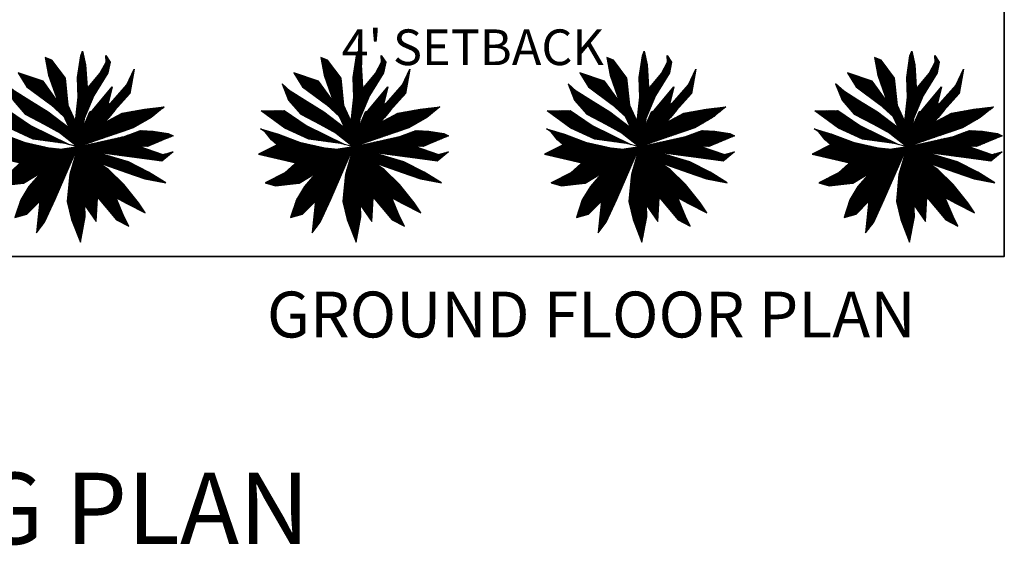
# Model space of a CAD drawing. Units: inches. Extents: x 1986 to 21484, y -1816 to 2016.
# Tile 2 of 85: x 2209 to 2402, y 1010 to 1113. Entities that reach past the tile are written whole.
import ezdxf

# ---------------------------------------------------------------- set-up
doc = ezdxf.new("R2010")
doc.units = ezdxf.units.IN
for name, color, linetype, lineweight in [('A-ANNO-TEXT', 7, 'Continuous', 18), ('C-PROP', 7, 'Continuous', 35), ('L-PLNT', 84, 'Continuous', 13), ('vfolhas', 114, 'Continuous', 5)]:
    doc.layers.add(name, color=color, linetype=linetype, lineweight=lineweight)
for name, color, linetype in [('vfolha', 72, 'Continuous'), ('vfolha2', 110, 'Continuous'), ('vfolhas2', 102, 'Continuous')]:
    doc.layers.add(name, color=color, linetype=linetype)
doc.styles.get("Standard").update_dxf_attribs({"font": 'arial.ttf'})
pattern_1 = [(45, (-2446.5133113, 50.986076), (-0.004419417382, 0.004419417382), [])]

# ---------------------------------------------------------------- blocks, each defined once
blk = doc.blocks.new('arbusto_PB_verde_grande')
at = {"layer": 'vfolha2'}
h = blk.add_hatch(dxfattribs=at)
h.set_pattern_fill('ANSI31', color=256, scale=0.05, style=0)
h.set_pattern_definition(pattern_1)
h.paths.add_polyline_path([(0.0294, 0.3565), (0.0003, 0.0905), (0.0263, -0.0393), (0.047, 0.0623), (0.0619, 0.0973), (0.0937, 0.2657), (0.0996, 0.4347), (0.0879, 0.6131), (0.0645, 0.7227), (0.0499, 0.6851), (0.0236, 0.5129)])
h.paths.add_polyline_path([(0.3011, 0.4379), (0.1423, 0.2487), (0.2669, 0.3002)])
h.paths.add_polyline_path([(0.38, 0.2282), (0.237, 0.1519), (0.1843, 0.0936), (0.1112, 0.0436), (0.0263, -0.0393), (0.2806, 0.0467), (0.3683, 0.078), (0.4676, 0.1124), (0.6107, 0.1938), (0.7159, 0.2782), (0.5581, 0.2595)])
h.paths.add_polyline_path([(0.561, -0.2944), (0.7275, -0.3257), (0.5902, -0.2412), (0.4296, -0.1598), (0.0263, -0.0393), (0.1492, -0.1411), (0.1884, -0.166), (0.415, -0.2444)])
h.paths.add_polyline_path([(-0.2743, -0.4478), (-0.3035, -0.7263), (-0.2392, -0.6417), (-0.1546, -0.4572), (0.0263, -0.0393), (-0.1633, -0.2538)])
h.paths.add_polyline_path([(-0.5196, -0.2474), (-0.6774, -0.3257), (-0.5956, -0.3507), (-0.4057, -0.3288), (-0.2101, -0.21), (0.0263, -0.0393), (-0.1487, -0.0659), (-0.3152, -0.091), (-0.4145, -0.1505)])
h.paths.add_polyline_path([(-0.5255, 0.2501), (-0.7095, 0.247), (-0.5196, 0.1093), (-0.3298, 0.0217), (-0.0757, -0.0128), (-0.0423, -0.0215), (-0.3502, 0.1312)])
h = blk.add_hatch(dxfattribs=at)
h.set_pattern_fill('ANSI31', color=256, scale=0.05, style=0)
h.set_pattern_definition(pattern_1)
h.paths.add_polyline_path([(-0.1896, 0.297), (-0.0855, 0.2019), (-0.1078, 0.2501), (-0.132, 0.3187), (-0.251, 0.4848), (-0.4495, 0.5505), (-0.3795, 0.4379)])
h.paths.add_polyline_path([(0.0791, -0.4071), (0.0821, -0.5063), (0.1726, -0.6355), (0.1843, -0.4415), (0.149, -0.2918), (0.0263, -0.0393), (0.0353, -0.2538)])
at = {"layer": 'vfolhas'}
h = blk.add_hatch(dxfattribs=at)
h.set_pattern_fill('ANSI31', color=256, scale=0.05, style=0)
h.set_pattern_definition(pattern_1)
h.paths.add_polyline_path([(-0.0728, 0.5067), (-0.1808, 0.6506), (-0.2334, 0.6725), (-0.2071, 0.5318), (-0.1078, 0.2501), (0.0263, -0.0393), (0.0003, 0.0905), (0.0082, 0.1624), (-0.0494, 0.2908)])
h.paths.add_polyline_path([(0.099, 0.4193), (0.0937, 0.2657), (0.0791, 0.1881), (0.1551, 0.369), (0.2661, 0.5505), (0.2836, 0.635), (0.2485, 0.6882), (0.2514, 0.635), (0.2018, 0.5443)])
h.paths.add_polyline_path([(0.1229, 0.2407), (0.047, 0.0623), (0.0263, -0.0393), (0.1112, 0.0436), (0.1843, 0.0936), (0.2748, 0.1938), (0.3215, 0.2532), (0.4413, 0.3847), (0.4763, 0.5787), (0.4179, 0.4535), (0.2894, 0.3095)])
h.paths.add_polyline_path([(0.5815, -0.0378), (0.7071, 0.0154), (0.7859, 0.0467), (0.748, 0.0655), (0.6282, 0.0842), (0.526, 0.0905), (0.3974, 0.0436), (0.0263, -0.0393), (0.2573, -0.0315), (0.4383, -0.0347)])
h.paths.add_polyline_path([(0.5202, -0.0365), (0.4383, -0.0347), (0.2573, -0.0315), (0.0263, -0.0393), (0.1796, -0.0852), (0.5377, -0.1317), (0.6954, -0.1536), (0.7859, -0.0785), (0.7041, -0.1004)])
h.paths.add_polyline_path([(0.2719, -0.2193), (0.1492, -0.1411), (0.0263, -0.0393), (0.1579, -0.3101), (0.2952, -0.4258), (0.4179, -0.4916), (0.564, -0.5667), (0.5114, -0.4853), (0.3946, -0.3414)])
h.paths.add_polyline_path([(-0.0582, -0.4759), (-0.0231, -0.6198), (0.047, -0.8013), (0.0849, -0.5979), (0.0791, -0.4071), (0.0353, -0.2538), (0.0263, -0.0393), (-0.0377, -0.26)])
h.paths.add_polyline_path([(-0.2422, 0.1405), (-0.1107, 0.0686), (0.0263, -0.0393), (-0.0423, 0.1087), (-0.2101, 0.2376), (-0.3649, 0.3314), (-0.4787, 0.4034), (-0.543, 0.4629), (-0.4904, 0.3314), (-0.3941, 0.2219)])
h = blk.add_hatch(dxfattribs=at)
h.set_pattern_fill('ANSI31', color=256, scale=0.05, style=0)
h.set_pattern_definition(pattern_1)
h.paths.add_polyline_path([(-0.5722, 0.0623), (-0.7153, 0.103), (-0.6774, 0.0811), (-0.6277, 0.0154), (-0.5635, -0.041), (-0.2646, -0.0834), (-0.1487, -0.0659), (-0.1015, -0.0588), (-0.2042, -0.0472), (-0.4028, -0.0034)])
h.paths.add_polyline_path([(-0.5635, -0.041), (-0.5828, -0.024), (-0.7299, -0.0973), (-0.4334, -0.1679), (-0.4145, -0.1505), (-0.3152, -0.091), (-0.2646, -0.0834)])
h.paths.add_polyline_path([(-0.2769, -0.4727), (-0.2743, -0.4478), (-0.1633, -0.2538), (0.0263, -0.0393), (-0.2101, -0.21), (-0.2672, -0.2447), (-0.3649, -0.357), (-0.4291, -0.4634), (-0.4759, -0.6043), (-0.3795, -0.576)])
h = blk.add_hatch(dxfattribs=at)
h.set_pattern_fill('ANSI31', color=256, scale=0.05, style=0)
h.set_pattern_definition(pattern_1)
h.paths.add_polyline_path([(0.3361, -0.623), (0.4325, -0.6731), (0.3946, -0.5948), (0.3303, -0.4446), (0.2952, -0.4258), (0.1579, -0.3101), (0.149, -0.2918), (0.1843, -0.4415)])
at = {"layer": 'vfolha'}
for p, q in [((0.0263, -0.0393), (-0.1487, -0.0659)), ((0.0263, -0.0393), (-0.0377, -0.26)), ((0.0353, -0.2538), (0.0263, -0.0393)), ((0.5202, -0.0365), (0.7041, -0.1004)), ((0.7859, -0.0785), (0.6954, -0.1536)), ((0.7041, -0.1004), (0.7859, -0.0785)), ((0.5377, -0.1317), (0.1796, -0.0852)), ((0.6954, -0.1536), (0.5377, -0.1317)), ((0.3946, -0.3414), (0.2719, -0.2193)), ((-0.2672, -0.2447), (-0.3649, -0.357)), ((-0.0377, -0.26), (-0.0582, -0.4759)), ((0.0791, -0.4071), (0.0353, -0.2538)), ((0.1579, -0.3101), (0.2952, -0.4258)), ((0.5114, -0.4853), (0.3946, -0.3414)), ((0.0849, -0.5979), (0.0791, -0.4071)), ((0.2952, -0.4258), (0.4179, -0.4916)), ((0.4179, -0.4916), (0.564, -0.5667)), ((0.564, -0.5667), (0.5114, -0.4853)), ((-0.0231, -0.6198), (0.047, -0.8013)), ((0.047, -0.8013), (0.0849, -0.5979))]:
    blk.add_line(p, q, dxfattribs=at)
at = {"layer": 'vfolha2'}
for p, q in [((0.0499, 0.6851), (0.0645, 0.7227)), ((0.0645, 0.7227), (0.0879, 0.6131)), ((0.0236, 0.5129), (0.0499, 0.6851)), ((-0.4495, 0.5505), (-0.3795, 0.4379)), ((-0.251, 0.4848), (-0.4495, 0.5505)), ((0.0879, 0.6131), (0.0996, 0.4347)), ((-0.132, 0.3187), (-0.251, 0.4848)), ((0.0294, 0.3565), (0.0236, 0.5129)), ((-0.3795, 0.4379), (-0.1896, 0.297)), ((0.0996, 0.4347), (0.0937, 0.2657)), ((0.1434, 0.2501), (0.3011, 0.4379)), ((0.3011, 0.4379), (0.2661, 0.297)), ((0.0003, 0.0905), (0.0294, 0.3565)), ((-0.7095, 0.247), (-0.5255, 0.2501)), ((-0.5196, 0.1093), (-0.7095, 0.247)), ((-0.5255, 0.2501), (-0.3502, 0.1312)), ((-0.1896, 0.297), (-0.0822, 0.1989)), ((0.38, 0.2282), (0.5581, 0.2595)), ((0.5581, 0.2595), (0.7159, 0.2782)), ((0.7159, 0.2782), (0.6107, 0.1938)), ((0.237, 0.1519), (0.38, 0.2282)), ((0.6107, 0.1938), (0.4676, 0.1124)), ((-0.3298, 0.0217), (-0.5196, 0.1093)), ((-0.3502, 0.1312), (-0.0423, -0.0215)), ((0.0263, -0.0393), (0.0003, 0.0905)), ((-0.0757, -0.0128), (-0.3298, 0.0217)), ((0.2806, 0.0467), (0.0263, -0.0393)), ((0.3683, 0.078), (0.2806, 0.0467)), ((-0.1487, -0.0659), (-0.3152, -0.091)), ((-0.2101, -0.21), (0.0263, -0.0393)), ((0.0263, -0.0393), (-0.1633, -0.2538)), ((-0.1546, -0.4572), (0.0263, -0.0393)), ((0.4296, -0.1598), (0.0263, -0.0393)), ((0.0263, -0.0393), (0.1579, -0.3101)), ((-0.4145, -0.1505), (-0.5196, -0.2474)), ((-0.3152, -0.091), (-0.4145, -0.1505)), ((-0.4057, -0.3288), (-0.2101, -0.21)), ((0.1884, -0.166), (0.415, -0.2444)), ((0.5902, -0.2412), (0.4296, -0.1598)), ((-0.5196, -0.2474), (-0.6774, -0.3257)), ((-0.1633, -0.2538), (-0.2743, -0.4478)), ((0.1843, -0.4415), (0.149, -0.2918)), ((0.415, -0.2444), (0.561, -0.2944)), ((0.561, -0.2944), (0.7275, -0.3257)), ((0.7275, -0.3257), (0.5902, -0.2412)), ((-0.6774, -0.3257), (-0.5956, -0.3507)), ((-0.5956, -0.3507), (-0.4057, -0.3288)), ((-0.2743, -0.4478), (-0.3035, -0.7263)), ((0.1726, -0.6355), (0.1843, -0.4415)), ((0.0821, -0.5063), (0.1726, -0.6355)), ((-0.3035, -0.7263), (-0.2392, -0.6417))]:
    blk.add_line(p, q, dxfattribs=at)
at = {"layer": 'vfolhas2'}
for p, q in [((-0.2334, 0.6725), (-0.2071, 0.5318)), ((-0.1808, 0.6506), (-0.2334, 0.6725)), ((-0.0728, 0.5067), (-0.1808, 0.6506)), ((0.2018, 0.5443), (0.2514, 0.635)), ((0.2514, 0.635), (0.2485, 0.6882)), ((0.2485, 0.6882), (0.2836, 0.635)), ((0.2836, 0.635), (0.2661, 0.5505)), ((0.2661, 0.5505), (0.1551, 0.369)), ((0.4179, 0.4535), (0.4763, 0.5787)), ((0.4763, 0.5787), (0.4413, 0.3847)), ((-0.2071, 0.5318), (-0.1078, 0.2501)), ((-0.0494, 0.2908), (-0.0728, 0.5067)), ((0.099, 0.4193), (0.2018, 0.5443)), ((-0.543, 0.4629), (-0.4904, 0.3314)), ((-0.4787, 0.4034), (-0.543, 0.4629)), ((-0.3649, 0.3314), (-0.4787, 0.4034)), ((0.2894, 0.3095), (0.4179, 0.4535)), ((-0.4904, 0.3314), (-0.3941, 0.2219)), ((-0.2101, 0.2376), (-0.3649, 0.3314)), ((0.1551, 0.369), (0.078, 0.1855)), ((0.4413, 0.3847), (0.3215, 0.2532)), ((-0.0423, 0.1087), (-0.2101, 0.2376)), ((-0.1078, 0.2501), (0.0263, -0.0393)), ((0.0082, 0.1624), (-0.0494, 0.2908)), ((0.047, 0.0623), (0.1229, 0.2407)), ((0.0937, 0.2657), (0.0619, 0.0973)), ((0.1229, 0.2407), (0.2894, 0.3095)), ((0.3215, 0.2532), (0.2748, 0.1938)), ((-0.3941, 0.2219), (-0.2422, 0.1405)), ((0.2748, 0.1938), (0.1843, 0.0936)), ((-0.6774, 0.0811), (-0.7153, 0.103)), ((-0.7153, 0.103), (-0.5722, 0.0623)), ((-0.6277, 0.0154), (-0.6774, 0.0811)), ((-0.2422, 0.1405), (-0.1107, 0.0686)), ((0.1843, 0.0936), (0.1112, 0.0436)), ((0.4676, 0.1124), (0.3683, 0.078)), ((0.3974, 0.0436), (0.526, 0.0905)), ((0.526, 0.0905), (0.6282, 0.0842)), ((0.6282, 0.0842), (0.748, 0.0655)), ((-0.5635, -0.041), (-0.6277, 0.0154)), ((-0.5722, 0.0623), (-0.4028, -0.0034)), ((-0.1107, 0.0686), (0.0263, -0.0393)), ((0.0263, -0.0393), (0.047, 0.0623)), ((0.0263, -0.0393), (0.3974, 0.0436)), ((0.1112, 0.0436), (0.0263, -0.0393)), ((0.7071, 0.0154), (0.5815, -0.0378)), ((0.7859, 0.0467), (0.7071, 0.0154)), ((0.748, 0.0655), (0.7859, 0.0467)), ((-0.5828, -0.024), (-0.7299, -0.0973)), ((-0.2646, -0.0834), (-0.5635, -0.041)), ((-0.4028, -0.0034), (-0.2042, -0.0472)), ((-0.2042, -0.0472), (-0.0983, -0.0591)), ((0.0263, -0.0393), (-0.0757, -0.0128)), ((0.2573, -0.0315), (0.0263, -0.0393)), ((0.1492, -0.1411), (0.0263, -0.0393)), ((0.4383, -0.0347), (0.2573, -0.0315)), ((0.5815, -0.0378), (0.4383, -0.0347)), ((-0.7299, -0.0973), (-0.4334, -0.1679)), ((0.2719, -0.2193), (0.1492, -0.1411)), ((-0.3649, -0.357), (-0.4291, -0.4634)), ((-0.4291, -0.4634), (-0.4759, -0.6043)), ((-0.2392, -0.6417), (-0.1546, -0.4572)), ((0.1843, -0.4415), (0.3361, -0.623)), ((0.3946, -0.5948), (0.329, -0.4417)), ((-0.3795, -0.576), (-0.2769, -0.4727)), ((-0.0582, -0.4759), (-0.0231, -0.6198)), ((-0.4759, -0.6043), (-0.3795, -0.576)), ((0.3361, -0.623), (0.4325, -0.6731)), ((0.4325, -0.6731), (0.3946, -0.5948))]:
    blk.add_line(p, q, dxfattribs=at)

msp = doc.modelspace()

# ---------------------------------------------------------------- linework, layer by layer
at = {"layer": 'C-PROP'}
msp.add_lwpolyline([(2042.31, 1900.75), (2402.31, 1900.75), (2402.31, 1066.75), (2042.31, 1066.75)], close=True, dxfattribs=at)

# ---------------------------------------------------------------- block references
at = {"layer": 'L-PLNT', "xscale": 24.60366729364114, "yscale": 24.60366729364114, "zscale": 24.60366729364114}
for p in [(2219.84, 1089.23), (2273.93, 1089.23), (2330.05, 1089.23), (2382.57, 1089.23)]:
    msp.add_blockref('arbusto_PB_verde_grande', p, dxfattribs=at)

# ---------------------------------------------------------------- texts
at = {"layer": 'A-ANNO-TEXT', "attachment_point": 1}
for s, width, insert, char_height in [("{\\fTimes New Roman|b0|i0|c0|p18;4' SETBACK}", 105.6127, (2272.25, 1111.29), 7), ('{\\fTimes New Roman|b0|i0|c0|p18;GROUND FLOOR PLAN}', 226.7688, (2257.6, 1059.84), 9), ('{\\fTimes New Roman|b0|i0|c0|p18;WEST FACING PLAN}', 226.7688, (2091.76, 1024.3), 14)]:
    msp.add_mtext_dynamic_manual_height_columns(s, width=width, gutter_width=12.5, heights=[0], dxfattribs=dict(at, insert=insert, char_height=char_height))

doc.saveas('drawing.dxf')
